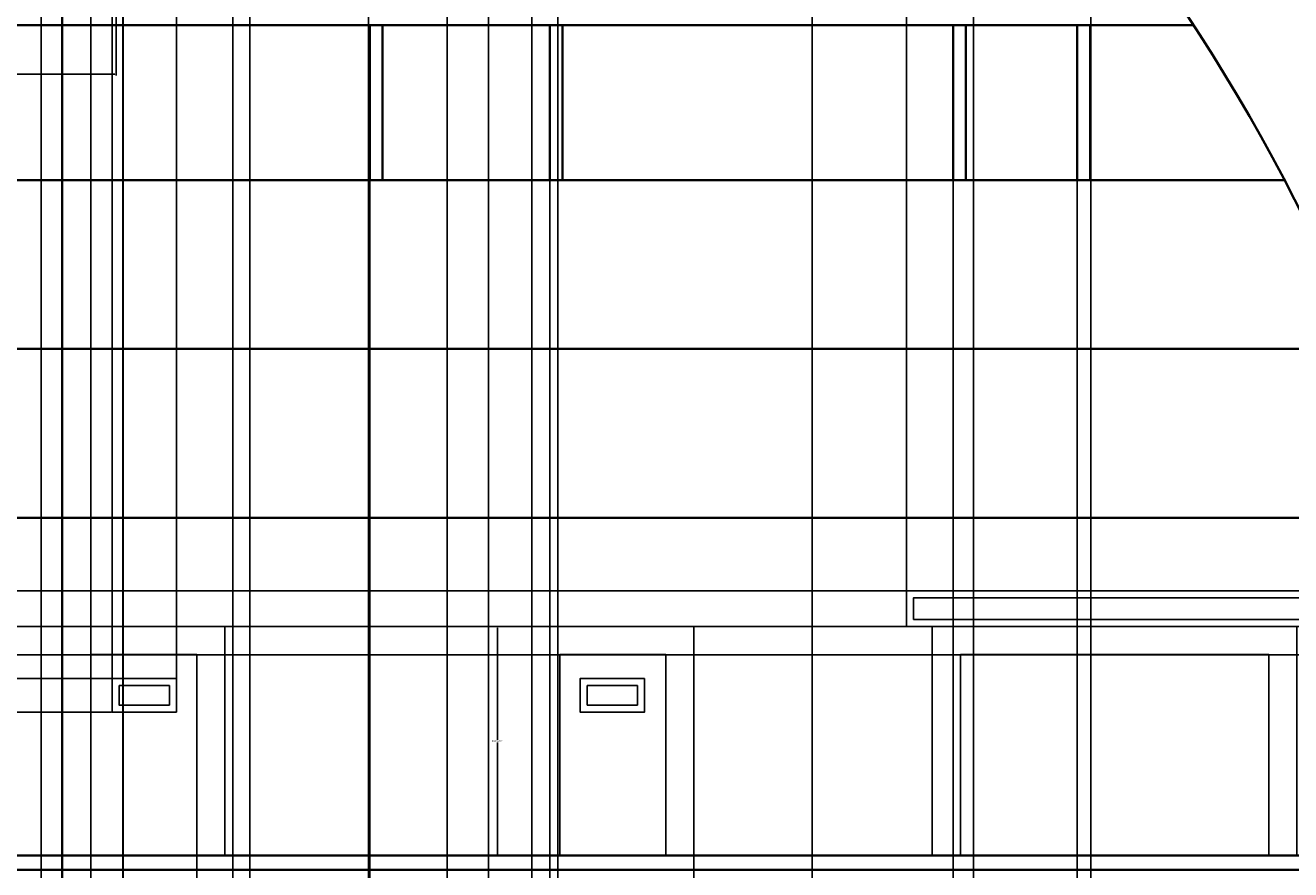
# Model space of a CAD drawing. Units: inches. Extents: x -19 to 408, y -26 to 603.
# Tile 3 of 7: x 137 to 317, y 169 to 289. Entities that reach past the tile are written whole.
import ezdxf

# ---------------------------------------------------------------- set-up
doc = ezdxf.new("R2010")
doc.units = ezdxf.units.IN
doc.header["$MEASUREMENT"] = 0
for name, color, linetype, lineweight in [('A-ANNO-DIMS', 2, 'Continuous', 18), ('A-DOOR', 3, 'Continuous', 25), ('A-ELEV', 7, 'Continuous', 35), ('A-GLAZ', 4, 'Continuous', 25)]:
    doc.layers.add(name, color=color, linetype=linetype, lineweight=lineweight)
doc.styles.get("Standard").update_dxf_attribs({"font": 'arial.ttf'})
doc.dimstyles.get("Standard").update_dxf_attribs({"dimtxt": 0.18, "dimasz": 0.18, "dimexe": 0.18, "dimexo": 0.0625, "dimgap": 0.09, "dimtad": 0, "dimtih": 1, "dimtoh": 1, "dimdec": 4, "dimzin": 0, "dimdsep": 46, "dimtxsty": 'Standard', "dimcen": 0.09, "dimadec": 0, "dimazin": 0, "dimtfac": 1, "dimtdec": 4, "dimtofl": 0, "dimtmove": 0, "dimatfit": 3, "dimfxl": 1, "dimtolj": 1, "dimtzin": 0, "dimarcsym": 0})

# ---------------------------------------------------------------- blocks, each defined once
blk = doc.blocks.new('WIN-1200')
for points in [[(0, 32.56), (59.66, 32.56), (59.66, 37.64), (0, 37.64)], [(1, 33.56), (58.66, 33.56), (58.66, 36.64), (1, 36.64)]]:
    blk.add_lwpolyline(points, close=True)
for points in [[(4.17, 0), (4.17, 32.56), (55.99, 32.56), (55.99, 0)], [(8.17, 0), (8.17, 28.56), (51.99, 28.56), (51.99, 0)]]:
    blk.add_lwpolyline(points)
blk = doc.blocks.new('DOOR-600')
for points in [[(0, 0), (0, 32.56), (23.06, 32.56), (23.06, 0)], [(4, 0), (4, 28.56), (19.06, 28.56), (19.06, 0)]]:
    blk.add_lwpolyline(points)
for points in [[(7.03, 25.16), (16.18, 25.16), (16.18, 20.4), (7.03, 20.4)], [(8.03, 24.16), (15.18, 24.16), (15.18, 21.4), (8.03, 21.4)]]:
    blk.add_lwpolyline(points, close=True)
blk = doc.blocks.new('RAIL-POST')
blk.add_lwpolyline([(0, 22), (1.83, 22), (1.83, 0), (0, 0)], close=True)
blk = doc.blocks.new('*D4')
at = {"layer": 'A-ANNO-DIMS', "color": 0, "lineweight": -2, "transparency": 16777216}
for p, q in [((89.99, 291.08), (89.99, 282.02)), ((149.65, 291.08), (149.65, 282.02)), ((90.17, 282.2), (118.7, 282.2)), ((149.47, 282.2), (120.94, 282.2))]:
    blk.add_line(p, q, dxfattribs=at)
at = {"layer": 'A-ANNO-DIMS', "color": 0, "transparency": 16777216}
for points in [[(90.17, 282.23), (90.17, 282.17), (89.99, 282.2)], [(149.47, 282.23), (149.47, 282.17), (149.65, 282.2)]]:
    blk.add_solid(points, dxfattribs=at)
at = {"layer": 'Defpoints', "color": 0, "transparency": 16777216}
for p in [(89.99, 291.15), (149.65, 291.15), (149.65, 282.2)]:
    blk.add_point(p, dxfattribs=at)
at = {"layer": 'A-ANNO-DIMS', "color": 0, "transparency": 16777216, "insert": (119.82, 282.2), "char_height": 0.18, "attachment_point": 5}
blk.add_mtext('\\A1;WINDOW 60 TYP.', dxfattribs=at)
blk = doc.blocks.new('*D6')
at = {"layer": 'A-ANNO-DIMS', "color": 0, "lineweight": -2, "transparency": 16777216}
for p, q in [((208.65, 203.7), (203.65, 203.7)), ((203.83, 203.52), (203.83, 187.61)), ((203.83, 171.33), (203.83, 187.24)), ((208.65, 171.15), (203.65, 171.15))]:
    blk.add_line(p, q, dxfattribs=at)
at = {"layer": 'A-ANNO-DIMS', "color": 0, "transparency": 16777216}
for points in [[(203.8, 203.52), (203.86, 203.52), (203.83, 203.7)], [(203.8, 171.33), (203.86, 171.33), (203.83, 171.15)]]:
    blk.add_solid(points, dxfattribs=at)
at = {"layer": 'Defpoints', "color": 0, "transparency": 16777216}
for p in [(203.83, 203.7), (208.71, 203.7), (208.71, 171.15)]:
    blk.add_point(p, dxfattribs=at)
at = {"layer": 'A-ANNO-DIMS', "color": 0, "transparency": 16777216, "insert": (203.83, 187.43), "char_height": 0.18, "attachment_point": 5}
blk.add_mtext('\\A1;DOOR 33 TYP.', dxfattribs=at)
blk = doc.blocks.new('*D7')
at = {"layer": 'A-ANNO-DIMS', "color": 0, "lineweight": -2, "transparency": 16777216}
for p, q in [((208.71, 171.08), (208.71, 166.08)), ((231.77, 171.08), (231.77, 166.08)), ((208.89, 166.26), (219.71, 166.26)), ((231.59, 166.26), (220.77, 166.26))]:
    blk.add_line(p, q, dxfattribs=at)
at = {"layer": 'A-ANNO-DIMS', "color": 0, "transparency": 16777216}
for points in [[(208.89, 166.29), (208.89, 166.23), (208.71, 166.26)], [(231.59, 166.29), (231.59, 166.23), (231.77, 166.26)]]:
    blk.add_solid(points, dxfattribs=at)
at = {"layer": 'Defpoints', "color": 0, "transparency": 16777216}
for p in [(208.71, 171.15), (231.77, 171.15), (208.71, 166.26)]:
    blk.add_point(p, dxfattribs=at)
at = {"layer": 'A-ANNO-DIMS', "color": 0, "transparency": 16777216, "insert": (220.24, 166.26), "char_height": 0.18, "attachment_point": 5}
blk.add_mtext('\\A1;23 TYP.', dxfattribs=at)
blk = doc.blocks.new('*D27')
at = {"layer": 'A-ANNO-DIMS', "color": 0, "lineweight": -2, "transparency": 16777216}
for p, q in [((288.17, 123.21), (288.17, 602.9)), ((288.35, 602.72), (324.05, 602.72)), ((360.39, 602.72), (324.69, 602.72)), ((360.57, 123.21), (360.57, 602.9))]:
    blk.add_line(p, q, dxfattribs=at)
at = {"layer": 'A-ANNO-DIMS', "color": 0, "transparency": 16777216}
for points in [[(288.35, 602.75), (288.35, 602.69), (288.17, 602.72)], [(360.39, 602.75), (360.39, 602.69), (360.57, 602.72)]]:
    blk.add_solid(points, dxfattribs=at)
at = {"layer": 'Defpoints', "color": 0, "transparency": 16777216}
for p in [(360.57, 602.72), (288.17, 123.15), (360.57, 123.15)]:
    blk.add_point(p, dxfattribs=at)
at = {"layer": 'A-ANNO-DIMS', "color": 0, "transparency": 16777216, "insert": (324.37, 602.72), "char_height": 0.18, "attachment_point": 5}
blk.add_mtext('\\A1;72.4', dxfattribs=at)
blk = doc.blocks.new('*D30')
at = {"layer": 'A-ANNO-DIMS', "color": 0, "lineweight": -2, "transparency": 16777216}
for p, q in [((360.57, 411.08), (360.57, -25.93)), ((185.52, 387.08), (185.52, -25.93)), ((185.7, -25.75), (272.59, -25.75)), ((360.39, -25.75), (273.5, -25.75))]:
    blk.add_line(p, q, dxfattribs=at)
at = {"layer": 'A-ANNO-DIMS', "color": 0, "transparency": 16777216}
for points in [[(185.7, -25.72), (185.7, -25.78), (185.52, -25.75)], [(360.39, -25.72), (360.39, -25.78), (360.57, -25.75)]]:
    blk.add_solid(points, dxfattribs=at)
at = {"layer": 'Defpoints', "color": 0, "transparency": 16777216}
for p in [(360.57, 411.15), (185.52, 387.15), (360.57, -25.75)]:
    blk.add_point(p, dxfattribs=at)
at = {"layer": 'A-ANNO-DIMS', "color": 0, "transparency": 16777216, "insert": (273.05, -25.75), "char_height": 0.18, "attachment_point": 5}
blk.add_mtext('\\A1;175.05', dxfattribs=at)
blk = doc.blocks.new('*D36')
at = {"layer": 'A-ANNO-DIMS', "color": 0, "lineweight": -2, "transparency": 16777216}
for p, q in [((52.15, 203.77), (52.15, 602.9)), ((52.33, 602.72), (96.69, 602.72)), ((141.84, 602.72), (97.48, 602.72)), ((142.02, 171.21), (142.02, 602.9))]:
    blk.add_line(p, q, dxfattribs=at)
at = {"layer": 'A-ANNO-DIMS', "color": 0, "transparency": 16777216}
for points in [[(52.33, 602.75), (52.33, 602.69), (52.15, 602.72)], [(141.84, 602.75), (141.84, 602.69), (142.02, 602.72)]]:
    blk.add_solid(points, dxfattribs=at)
at = {"layer": 'Defpoints', "color": 0, "transparency": 16777216}
for p in [(142.02, 602.72), (52.15, 203.7), (142.02, 171.15)]:
    blk.add_point(p, dxfattribs=at)
at = {"layer": 'A-ANNO-DIMS', "color": 0, "transparency": 16777216, "insert": (97.09, 602.72), "char_height": 0.18, "attachment_point": 5}
blk.add_mtext('\\A1;89.87', dxfattribs=at)
blk = doc.blocks.new('*D37')
at = {"layer": 'A-ANNO-DIMS', "color": 0, "lineweight": -2, "transparency": 16777216}
for p, q in [((142.02, 171.21), (142.02, 602.9)), ((142.2, 602.72), (174.97, 602.72)), ((208.53, 602.72), (175.76, 602.72)), ((208.71, 171.21), (208.71, 602.9))]:
    blk.add_line(p, q, dxfattribs=at)
at = {"layer": 'A-ANNO-DIMS', "color": 0, "transparency": 16777216}
for points in [[(142.2, 602.75), (142.2, 602.69), (142.02, 602.72)], [(208.53, 602.75), (208.53, 602.69), (208.71, 602.72)]]:
    blk.add_solid(points, dxfattribs=at)
at = {"layer": 'Defpoints', "color": 0, "transparency": 16777216}
for p in [(208.71, 602.72), (142.02, 171.15), (208.71, 171.15)]:
    blk.add_point(p, dxfattribs=at)
at = {"layer": 'A-ANNO-DIMS', "color": 0, "transparency": 16777216, "insert": (175.37, 602.72), "char_height": 0.18, "attachment_point": 5}
blk.add_mtext('\\A1;66.69', dxfattribs=at)
blk = doc.blocks.new('*D38')
at = {"layer": 'A-ANNO-DIMS', "color": 0, "lineweight": -2, "transparency": 16777216}
for p, q in [((208.71, 171.21), (208.71, 602.9)), ((208.89, 602.72), (234.95, 602.72)), ((261.81, 602.72), (235.74, 602.72)), ((261.99, 203.77), (261.99, 602.9))]:
    blk.add_line(p, q, dxfattribs=at)
at = {"layer": 'A-ANNO-DIMS', "color": 0, "transparency": 16777216}
for points in [[(208.89, 602.75), (208.89, 602.69), (208.71, 602.72)], [(261.81, 602.75), (261.81, 602.69), (261.99, 602.72)]]:
    blk.add_solid(points, dxfattribs=at)
at = {"layer": 'Defpoints', "color": 0, "transparency": 16777216}
for p in [(261.99, 602.72), (261.99, 203.7), (208.71, 171.15)]:
    blk.add_point(p, dxfattribs=at)
at = {"layer": 'A-ANNO-DIMS', "color": 0, "transparency": 16777216, "insert": (235.35, 602.72), "char_height": 0.18, "attachment_point": 5}
blk.add_mtext('\\A1;53.28', dxfattribs=at)
blk = doc.blocks.new('*D50')
at = {"layer": 'A-ANNO-DIMS', "color": 0, "lineweight": -2, "transparency": 16777216}
for p, q in [((104.21, 199.7), (407.65, 199.7)), ((407.47, 199.52), (407.47, 185.61)), ((407.47, 171.33), (407.47, 185.24)), ((104.21, 171.15), (407.65, 171.15))]:
    blk.add_line(p, q, dxfattribs=at)
at = {"layer": 'A-ANNO-DIMS', "color": 0, "transparency": 16777216}
for points in [[(407.44, 199.52), (407.5, 199.52), (407.47, 199.7)], [(407.44, 171.33), (407.5, 171.33), (407.47, 171.15)]]:
    blk.add_solid(points, dxfattribs=at)
at = {"layer": 'Defpoints', "color": 0, "transparency": 16777216}
for p in [(104.14, 199.7), (407.47, 199.7), (104.14, 171.15)]:
    blk.add_point(p, dxfattribs=at)
at = {"layer": 'A-ANNO-DIMS', "color": 0, "transparency": 16777216, "insert": (407.47, 185.43), "char_height": 0.18, "attachment_point": 5}
blk.add_mtext('\\A1;28.557', dxfattribs=at)
blk = doc.blocks.new('*D51')
at = {"layer": 'A-ANNO-DIMS', "color": 0, "lineweight": -2, "transparency": 16777216}
for p, q in [((108.207069, 203.703989), (407.651202, 203.703989)), ((407.471202, 203.523989), (407.471202, 201.883989)), ((407.471202, 199.883989), (407.471202, 201.523989)), ((104.207069, 199.703989), (407.651202, 199.703989))]:
    blk.add_line(p, q, dxfattribs=at)
at = {"layer": 'A-ANNO-DIMS', "color": 0, "transparency": 16777216}
for points in [[(407.441202, 203.523989), (407.501202, 203.523989), (407.471202, 203.703989)], [(407.441202, 199.883989), (407.501202, 199.883989), (407.471202, 199.703989)]]:
    blk.add_solid(points, dxfattribs=at)
at = {"layer": 'Defpoints', "color": 0, "transparency": 16777216}
for p in [(108.144569, 203.703989), (407.471202, 203.703989), (104.144569, 199.703989)]:
    blk.add_point(p, dxfattribs=at)
at = {"layer": 'A-ANNO-DIMS', "color": 0, "transparency": 16777216, "insert": (407.471202, 201.703989), "char_height": 0.18, "attachment_point": 5}
blk.add_mtext('\\A1;4', dxfattribs=at)
blk = doc.blocks.new('*D52')
at = {"layer": 'A-ANNO-DIMS', "color": 0, "lineweight": -2, "transparency": 16777216}
for p, q in [((111.87, 208.79), (407.65, 208.79)), ((407.47, 208.61), (407.47, 206.43)), ((407.47, 203.88), (407.47, 206.07)), ((111.87, 203.7), (407.65, 203.7))]:
    blk.add_line(p, q, dxfattribs=at)
at = {"layer": 'A-ANNO-DIMS', "color": 0, "transparency": 16777216}
for points in [[(407.44, 208.61), (407.5, 208.61), (407.47, 208.79)], [(407.44, 203.88), (407.5, 203.88), (407.47, 203.7)]]:
    blk.add_solid(points, dxfattribs=at)
at = {"layer": 'Defpoints', "color": 0, "transparency": 16777216}
for p in [(111.81, 208.79), (407.47, 208.79), (111.81, 203.7)]:
    blk.add_point(p, dxfattribs=at)
at = {"layer": 'A-ANNO-DIMS', "color": 0, "transparency": 16777216, "insert": (407.47, 206.25), "char_height": 0.18, "attachment_point": 5}
blk.add_mtext('\\A1;5.086', dxfattribs=at)
blk = doc.blocks.new('*D53')
at = {"layer": 'A-ANNO-DIMS', "color": 0, "lineweight": -2, "transparency": 16777216}
for p, q in [((142.02, 171.08), (142.02, -25.93)), ((146.02, 171.08), (146.02, -25.93)), ((142.2, -25.75), (143.87, -25.75)), ((145.84, -25.75), (144.18, -25.75))]:
    blk.add_line(p, q, dxfattribs=at)
at = {"layer": 'A-ANNO-DIMS', "color": 0, "transparency": 16777216}
for points in [[(142.2, -25.72), (142.2, -25.78), (142.02, -25.75)], [(145.84, -25.72), (145.84, -25.78), (146.02, -25.75)]]:
    blk.add_solid(points, dxfattribs=at)
at = {"layer": 'Defpoints', "color": 0, "transparency": 16777216}
for p in [(142.02, 171.15), (146.02, 171.15), (146.02, -25.75)]:
    blk.add_point(p, dxfattribs=at)
at = {"layer": 'A-ANNO-DIMS', "color": 0, "transparency": 16777216, "insert": (144.02, -25.75), "char_height": 0.18, "attachment_point": 5}
blk.add_mtext('\\A1;4', dxfattribs=at)
blk = doc.blocks.new('*D54')
at = {"layer": 'A-ANNO-DIMS', "color": 0, "lineweight": -2, "transparency": 16777216}
for p, q in [((146.02, 171.08), (146.02, -25.93)), ((161.09, 171.08), (161.09, -25.93)), ((146.2, -25.75), (153.1, -25.75)), ((160.91, -25.75), (154.01, -25.75))]:
    blk.add_line(p, q, dxfattribs=at)
at = {"layer": 'A-ANNO-DIMS', "color": 0, "transparency": 16777216}
for points in [[(146.2, -25.72), (146.2, -25.78), (146.02, -25.75)], [(160.91, -25.72), (160.91, -25.78), (161.09, -25.75)]]:
    blk.add_solid(points, dxfattribs=at)
at = {"layer": 'Defpoints', "color": 0, "transparency": 16777216}
for p in [(146.02, 171.15), (161.09, 171.15), (161.09, -25.75)]:
    blk.add_point(p, dxfattribs=at)
at = {"layer": 'A-ANNO-DIMS', "color": 0, "transparency": 16777216, "insert": (153.56, -25.75), "char_height": 0.18, "attachment_point": 5}
blk.add_mtext('\\A1;15.064', dxfattribs=at)
blk = doc.blocks.new('*D55')
at = {"layer": 'A-ANNO-DIMS', "color": 0, "lineweight": -2, "transparency": 16777216}
for p, q in [((146.02, 199.77), (146.02, 602.9)), ((146.2, 602.72), (147.14, 602.72)), ((148.87, 602.72), (147.93, 602.72)), ((149.05, 196.37), (149.05, 602.9))]:
    blk.add_line(p, q, dxfattribs=at)
at = {"layer": 'A-ANNO-DIMS', "color": 0, "transparency": 16777216}
for points in [[(146.2, 602.75), (146.2, 602.69), (146.02, 602.72)], [(148.87, 602.75), (148.87, 602.69), (149.05, 602.72)]]:
    blk.add_solid(points, dxfattribs=at)
at = {"layer": 'Defpoints', "color": 0, "transparency": 16777216}
for p in [(149.05, 602.72), (146.02, 199.7), (149.05, 196.31)]:
    blk.add_point(p, dxfattribs=at)
at = {"layer": 'A-ANNO-DIMS', "color": 0, "transparency": 16777216, "insert": (147.54, 602.72), "char_height": 0.18, "attachment_point": 5}
blk.add_mtext('\\A1;3.029', dxfattribs=at)
blk = doc.blocks.new('*D56')
at = {"layer": 'A-ANNO-DIMS', "color": 0, "lineweight": -2, "transparency": 16777216}
for p, q in [((149.05, 196.37), (149.05, 602.9)), ((149.23, 602.72), (153.3, 602.72)), ((158.02, 602.72), (153.95, 602.72)), ((158.2, 196.37), (158.2, 602.9))]:
    blk.add_line(p, q, dxfattribs=at)
at = {"layer": 'A-ANNO-DIMS', "color": 0, "transparency": 16777216}
for points in [[(149.23, 602.75), (149.23, 602.69), (149.05, 602.72)], [(158.02, 602.75), (158.02, 602.69), (158.2, 602.72)]]:
    blk.add_solid(points, dxfattribs=at)
at = {"layer": 'Defpoints', "color": 0, "transparency": 16777216}
for p in [(158.2, 602.72), (149.05, 196.31), (158.2, 196.31)]:
    blk.add_point(p, dxfattribs=at)
at = {"layer": 'A-ANNO-DIMS', "color": 0, "transparency": 16777216, "insert": (153.63, 602.72), "char_height": 0.18, "attachment_point": 5}
blk.add_mtext('\\A1;9.15', dxfattribs=at)
blk = doc.blocks.new('*D57')
at = {"layer": 'A-ANNO-DIMS', "color": 0, "lineweight": -2, "transparency": 16777216}
for p, q in [((148.99, 196.31), (-18.88, 196.31)), ((-18.7, 196.13), (-18.7, 194.11)), ((-18.7, 191.73), (-18.7, 193.75)), ((148.99, 191.55), (-18.88, 191.55))]:
    blk.add_line(p, q, dxfattribs=at)
at = {"layer": 'A-ANNO-DIMS', "color": 0, "transparency": 16777216}
for points in [[(-18.73, 196.13), (-18.67, 196.13), (-18.7, 196.31)], [(-18.73, 191.73), (-18.67, 191.73), (-18.7, 191.55)]]:
    blk.add_solid(points, dxfattribs=at)
at = {"layer": 'Defpoints', "color": 0, "transparency": 16777216}
for p in [(-18.7, 196.31), (149.05, 196.31), (149.05, 191.55)]:
    blk.add_point(p, dxfattribs=at)
at = {"layer": 'A-ANNO-DIMS', "color": 0, "transparency": 16777216, "insert": (-18.7, 193.93), "char_height": 0.18, "attachment_point": 5}
blk.add_mtext('\\A1;4.756', dxfattribs=at)
blk = doc.blocks.new('*D58')
at = {"layer": 'A-ANNO-DIMS', "color": 0, "lineweight": -2, "transparency": 16777216}
for p, q in [((145.96, 199.7), (-18.88, 199.7)), ((-18.7, 199.52), (-18.7, 198.19)), ((148.99, 196.31), (-18.88, 196.31)), ((-18.7, 196.49), (-18.7, 197.82))]:
    blk.add_line(p, q, dxfattribs=at)
at = {"layer": 'A-ANNO-DIMS', "color": 0, "transparency": 16777216}
for points in [[(-18.73, 199.52), (-18.67, 199.52), (-18.7, 199.7)], [(-18.73, 196.49), (-18.67, 196.49), (-18.7, 196.31)]]:
    blk.add_solid(points, dxfattribs=at)
at = {"layer": 'Defpoints', "color": 0, "transparency": 16777216}
for p in [(-18.7, 199.7), (146.02, 199.7), (149.05, 196.31)]:
    blk.add_point(p, dxfattribs=at)
at = {"layer": 'A-ANNO-DIMS', "color": 0, "transparency": 16777216, "insert": (-18.7, 198), "char_height": 0.18, "attachment_point": 5}
blk.add_mtext('\\A1;3.398', dxfattribs=at)
blk = doc.blocks.new('*D59')
at = {"layer": 'A-ANNO-DIMS', "color": 0, "lineweight": -2, "transparency": 16777216}
for p, q in [((161.15, 199.7), (407.65, 199.7)), ((407.47, 199.52), (407.47, 185.61)), ((407.47, 171.33), (407.47, 185.24)), ((161.15, 171.15), (407.65, 171.15))]:
    blk.add_line(p, q, dxfattribs=at)
at = {"layer": 'A-ANNO-DIMS', "color": 0, "transparency": 16777216}
for points in [[(407.44, 199.52), (407.5, 199.52), (407.47, 199.7)], [(407.44, 171.33), (407.5, 171.33), (407.47, 171.15)]]:
    blk.add_solid(points, dxfattribs=at)
at = {"layer": 'Defpoints', "color": 0, "transparency": 16777216}
for p in [(161.09, 199.7), (407.47, 199.7), (161.09, 171.15)]:
    blk.add_point(p, dxfattribs=at)
at = {"layer": 'A-ANNO-DIMS', "color": 0, "transparency": 16777216, "insert": (407.47, 185.43), "char_height": 0.18, "attachment_point": 5}
blk.add_mtext('\\A1;28.557', dxfattribs=at)
blk = doc.blocks.new('*D62')
at = {"layer": 'A-ANNO-DIMS', "color": 0, "lineweight": -2, "transparency": 16777216}
for p, q in [((131.96, 267.08), (131.96, -25.93)), ((185.68, 267.08), (185.68, -25.93)), ((132.14, -25.75), (158.43, -25.75)), ((185.5, -25.75), (159.21, -25.75))]:
    blk.add_line(p, q, dxfattribs=at)
at = {"layer": 'A-ANNO-DIMS', "color": 0, "transparency": 16777216}
for points in [[(132.14, -25.72), (132.14, -25.78), (131.96, -25.75)], [(185.5, -25.72), (185.5, -25.78), (185.68, -25.75)]]:
    blk.add_solid(points, dxfattribs=at)
at = {"layer": 'Defpoints', "color": 0, "transparency": 16777216}
for p in [(131.96, 267.15), (185.68, 267.15), (185.68, -25.75)]:
    blk.add_point(p, dxfattribs=at)
at = {"layer": 'A-ANNO-DIMS', "color": 0, "transparency": 16777216, "insert": (158.82, -25.75), "char_height": 0.18, "attachment_point": 5}
blk.add_mtext('\\A1;53.72', dxfattribs=at)
blk = doc.blocks.new('*D63')
at = {"layer": 'A-ANNO-DIMS', "color": 0, "lineweight": -2, "transparency": 16777216}
for p, q in [((185.68, 267.08), (185.68, -25.93)), ((211.27, 267.08), (211.27, -25.93)), ((185.86, -25.75), (198.01, -25.75)), ((211.09, -25.75), (198.94, -25.75))]:
    blk.add_line(p, q, dxfattribs=at)
at = {"layer": 'A-ANNO-DIMS', "color": 0, "transparency": 16777216}
for points in [[(185.86, -25.72), (185.86, -25.78), (185.68, -25.75)], [(211.09, -25.72), (211.09, -25.78), (211.27, -25.75)]]:
    blk.add_solid(points, dxfattribs=at)
at = {"layer": 'Defpoints', "color": 0, "transparency": 16777216}
for p in [(185.68, 267.15), (211.27, 267.15), (211.27, -25.75)]:
    blk.add_point(p, dxfattribs=at)
at = {"layer": 'A-ANNO-DIMS', "color": 0, "transparency": 16777216, "insert": (198.47, -25.75), "char_height": 0.18, "attachment_point": 5}
blk.add_mtext('\\A1;25.584', dxfattribs=at)
blk = doc.blocks.new('*D64')
at = {"layer": 'A-ANNO-DIMS', "color": 0, "lineweight": -2, "transparency": 16777216}
for p, q in [((211.27, 267.08), (211.27, -25.93)), ((268.61, 267.08), (268.61, -25.93)), ((211.45, -25.75), (239.55, -25.75)), ((268.43, -25.75), (240.33, -25.75))]:
    blk.add_line(p, q, dxfattribs=at)
at = {"layer": 'A-ANNO-DIMS', "color": 0, "transparency": 16777216}
for points in [[(211.45, -25.72), (211.45, -25.78), (211.27, -25.75)], [(268.43, -25.72), (268.43, -25.78), (268.61, -25.75)]]:
    blk.add_solid(points, dxfattribs=at)
at = {"layer": 'Defpoints', "color": 0, "transparency": 16777216}
for p in [(211.27, 267.15), (268.61, 267.15), (268.61, -25.75)]:
    blk.add_point(p, dxfattribs=at)
at = {"layer": 'A-ANNO-DIMS', "color": 0, "transparency": 16777216, "insert": (239.94, -25.75), "char_height": 0.18, "attachment_point": 5}
blk.add_mtext('\\A1;57.34', dxfattribs=at)
blk = doc.blocks.new('*D65')
at = {"layer": 'A-ANNO-DIMS', "color": 0, "lineweight": -2, "transparency": 16777216}
for p, q in [((268.61, 267.08), (268.61, -25.93)), ((286.26, 267.08), (286.26, -25.93)), ((268.79, -25.75), (276.98, -25.75)), ((286.08, -25.75), (277.89, -25.75))]:
    blk.add_line(p, q, dxfattribs=at)
at = {"layer": 'A-ANNO-DIMS', "color": 0, "transparency": 16777216}
for points in [[(268.79, -25.72), (268.79, -25.78), (268.61, -25.75)], [(286.08, -25.72), (286.08, -25.78), (286.26, -25.75)]]:
    blk.add_solid(points, dxfattribs=at)
at = {"layer": 'Defpoints', "color": 0, "transparency": 16777216}
for p in [(268.61, 267.15), (286.26, 267.15), (286.26, -25.75)]:
    blk.add_point(p, dxfattribs=at)
at = {"layer": 'A-ANNO-DIMS', "color": 0, "transparency": 16777216, "insert": (277.43, -25.75), "char_height": 0.18, "attachment_point": 5}
blk.add_mtext('\\A1;17.644', dxfattribs=at)
blk = doc.blocks.new('*D70')
at = {"layer": 'A-ANNO-DIMS', "color": 0, "lineweight": -2, "transparency": 16777216}
for p, q in [((150.62, 387.08), (150.62, -25.93)), ((185.52, 387.08), (185.52, -25.93)), ((150.8, -25.75), (167.6, -25.75)), ((185.34, -25.75), (168.53, -25.75))]:
    blk.add_line(p, q, dxfattribs=at)
at = {"layer": 'A-ANNO-DIMS', "color": 0, "transparency": 16777216}
for points in [[(150.8, -25.72), (150.8, -25.78), (150.62, -25.75)], [(185.34, -25.72), (185.34, -25.78), (185.52, -25.75)]]:
    blk.add_solid(points, dxfattribs=at)
at = {"layer": 'Defpoints', "color": 0, "transparency": 16777216}
for p in [(150.62, 387.15), (185.52, 387.15), (185.52, -25.75)]:
    blk.add_point(p, dxfattribs=at)
at = {"layer": 'A-ANNO-DIMS', "color": 0, "transparency": 16777216, "insert": (168.07, -25.75), "char_height": 0.18, "attachment_point": 5}
blk.add_mtext('\\A1;34.906', dxfattribs=at)
blk = doc.blocks.new('*D73')
at = {"layer": 'A-ANNO-DIMS', "color": 0, "lineweight": -2, "transparency": 16777216}
for p, q in [((185.52, 411.08), (185.52, -25.93)), ((208.71, 411.08), (208.71, -25.93)), ((185.7, -25.75), (196.72, -25.75)), ((208.53, -25.75), (197.51, -25.75))]:
    blk.add_line(p, q, dxfattribs=at)
at = {"layer": 'A-ANNO-DIMS', "color": 0, "transparency": 16777216}
for points in [[(185.7, -25.72), (185.7, -25.78), (185.52, -25.75)], [(208.53, -25.72), (208.53, -25.78), (208.71, -25.75)]]:
    blk.add_solid(points, dxfattribs=at)
at = {"layer": 'Defpoints', "color": 0, "transparency": 16777216}
for p in [(185.52, 411.15), (208.71, 411.15), (208.71, -25.75)]:
    blk.add_point(p, dxfattribs=at)
at = {"layer": 'A-ANNO-DIMS', "color": 0, "transparency": 16777216, "insert": (197.12, -25.75), "char_height": 0.18, "attachment_point": 5}
blk.add_mtext('\\A1;23.19', dxfattribs=at)
blk = doc.blocks.new('*D75')
at = {"layer": 'A-ANNO-DIMS', "color": 0, "lineweight": -2, "transparency": 16777216}
for p, q in [((212.43, 507.08), (212.43, -25.93)), ((248.57, 507.08), (248.57, -25.93)), ((212.61, -25.75), (230.11, -25.75)), ((248.39, -25.75), (230.89, -25.75))]:
    blk.add_line(p, q, dxfattribs=at)
at = {"layer": 'A-ANNO-DIMS', "color": 0, "transparency": 16777216}
for points in [[(212.61, -25.72), (212.61, -25.78), (212.43, -25.75)], [(248.39, -25.72), (248.39, -25.78), (248.57, -25.75)]]:
    blk.add_solid(points, dxfattribs=at)
at = {"layer": 'Defpoints', "color": 0, "transparency": 16777216}
for p in [(212.43, 507.15), (248.57, 507.15), (248.57, -25.75)]:
    blk.add_point(p, dxfattribs=at)
at = {"layer": 'A-ANNO-DIMS', "color": 0, "transparency": 16777216, "insert": (230.5, -25.75), "char_height": 0.18, "attachment_point": 5}
blk.add_mtext('\\A1;36.14', dxfattribs=at)
blk = doc.blocks.new('*D76')
at = {"layer": 'A-ANNO-DIMS', "color": 0, "lineweight": -2, "transparency": 16777216}
for p, q in [((248.57, 507.08), (248.57, -25.93)), ((271.51, 507.08), (271.51, -25.93)), ((248.75, -25.75), (259.58, -25.75)), ((271.33, -25.75), (260.51, -25.75))]:
    blk.add_line(p, q, dxfattribs=at)
at = {"layer": 'A-ANNO-DIMS', "color": 0, "transparency": 16777216}
for points in [[(248.75, -25.72), (248.75, -25.78), (248.57, -25.75)], [(271.33, -25.72), (271.33, -25.78), (271.51, -25.75)]]:
    blk.add_solid(points, dxfattribs=at)
at = {"layer": 'Defpoints', "color": 0, "transparency": 16777216}
for p in [(248.57, 507.15), (271.51, 507.15), (271.51, -25.75)]:
    blk.add_point(p, dxfattribs=at)
at = {"layer": 'A-ANNO-DIMS', "color": 0, "transparency": 16777216, "insert": (260.04, -25.75), "char_height": 0.18, "attachment_point": 5}
blk.add_mtext('\\A1;22.944', dxfattribs=at)
blk = doc.blocks.new('*D77')
at = {"layer": 'A-ANNO-DIMS', "color": 0, "lineweight": -2, "transparency": 16777216}
for p, q in [((271.51, 507.08), (271.51, -25.93)), ((325.24, 507.08), (325.24, -25.93)), ((271.69, -25.75), (297.98, -25.75)), ((325.06, -25.75), (298.77, -25.75))]:
    blk.add_line(p, q, dxfattribs=at)
at = {"layer": 'A-ANNO-DIMS', "color": 0, "transparency": 16777216}
for points in [[(271.69, -25.72), (271.69, -25.78), (271.51, -25.75)], [(325.06, -25.72), (325.06, -25.78), (325.24, -25.75)]]:
    blk.add_solid(points, dxfattribs=at)
at = {"layer": 'Defpoints', "color": 0, "transparency": 16777216}
for p in [(271.51, 507.15), (325.24, 507.15), (325.24, -25.75)]:
    blk.add_point(p, dxfattribs=at)
at = {"layer": 'A-ANNO-DIMS', "color": 0, "transparency": 16777216, "insert": (298.38, -25.75), "char_height": 0.18, "attachment_point": 5}
blk.add_mtext('\\A1;53.72', dxfattribs=at)
blk = doc.blocks.new('*D83')
at = {"layer": 'A-ANNO-DIMS', "color": 0, "lineweight": -2, "transparency": 16777216}
for p, q in [((141.92, 491.44), (141.92, -25.93)), ((166.23, 491.44), (166.23, -25.93)), ((142.1, -25.75), (153.69, -25.75)), ((166.05, -25.75), (154.45, -25.75))]:
    blk.add_line(p, q, dxfattribs=at)
at = {"layer": 'A-ANNO-DIMS', "color": 0, "transparency": 16777216}
for points in [[(142.1, -25.72), (142.1, -25.78), (141.92, -25.75)], [(166.05, -25.72), (166.05, -25.78), (166.23, -25.75)]]:
    blk.add_solid(points, dxfattribs=at)
at = {"layer": 'Defpoints', "color": 0, "transparency": 16777216}
for p in [(141.92, 491.5), (166.23, 491.5), (166.23, -25.75)]:
    blk.add_point(p, dxfattribs=at)
at = {"layer": 'A-ANNO-DIMS', "color": 0, "transparency": 16777216, "insert": (154.07, -25.75), "char_height": 0.18, "attachment_point": 5}
blk.add_mtext('\\A1;24.31', dxfattribs=at)
blk = doc.blocks.new('*D84')
at = {"layer": 'A-ANNO-DIMS', "color": 0, "lineweight": -2, "transparency": 16777216}
for p, q in [((138.97, 531.28), (138.97, -25.93)), ((168.64, 531.28), (168.64, -25.93)), ((139.15, -25.75), (153.41, -25.75)), ((168.46, -25.75), (154.2, -25.75))]:
    blk.add_line(p, q, dxfattribs=at)
at = {"layer": 'A-ANNO-DIMS', "color": 0, "transparency": 16777216}
for points in [[(139.15, -25.72), (139.15, -25.78), (138.97, -25.75)], [(168.46, -25.72), (168.46, -25.78), (168.64, -25.75)]]:
    blk.add_solid(points, dxfattribs=at)
at = {"layer": 'Defpoints', "color": 0, "transparency": 16777216}
for p in [(138.97, 531.34), (168.64, 531.34), (168.64, -25.75)]:
    blk.add_point(p, dxfattribs=at)
at = {"layer": 'A-ANNO-DIMS', "color": 0, "transparency": 16777216, "insert": (153.81, -25.75), "char_height": 0.18, "attachment_point": 5}
blk.add_mtext('\\A1;29.67', dxfattribs=at)
blk = doc.blocks.new('*D95')
at = {"layer": 'A-ANNO-DIMS', "color": 0, "lineweight": -2, "transparency": 16777216}
for p, q in [((150.57, 85.97), (150.57, 602.9)), ((150.75, 602.72), (173.31, 602.72)), ((196.49, 602.72), (173.93, 602.72)), ((196.67, 85.97), (196.67, 602.9))]:
    blk.add_line(p, q, dxfattribs=at)
at = {"layer": 'A-ANNO-DIMS', "color": 0, "transparency": 16777216}
for points in [[(150.75, 602.75), (150.75, 602.69), (150.57, 602.72)], [(196.49, 602.75), (196.49, 602.69), (196.67, 602.72)]]:
    blk.add_solid(points, dxfattribs=at)
at = {"layer": 'Defpoints', "color": 0, "transparency": 16777216}
for p in [(196.67, 602.72), (150.57, 85.9), (196.67, 85.9)]:
    blk.add_point(p, dxfattribs=at)
at = {"layer": 'A-ANNO-DIMS', "color": 0, "transparency": 16777216, "insert": (173.62, 602.72), "char_height": 0.18, "attachment_point": 5}
blk.add_mtext('\\A1;46.1', dxfattribs=at)
blk = doc.blocks.new('*D96')
at = {"layer": 'A-ANNO-DIMS', "color": 0, "lineweight": -2, "transparency": 16777216}
for p, q in [((196.67, 85.97), (196.67, 602.9)), ((196.85, 602.72), (199.31, 602.72)), ((202.41, 602.72), (199.96, 602.72)), ((202.59, 85.97), (202.59, 602.9))]:
    blk.add_line(p, q, dxfattribs=at)
at = {"layer": 'A-ANNO-DIMS', "color": 0, "transparency": 16777216}
for points in [[(196.85, 602.75), (196.85, 602.69), (196.67, 602.72)], [(202.41, 602.75), (202.41, 602.69), (202.59, 602.72)]]:
    blk.add_solid(points, dxfattribs=at)
at = {"layer": 'Defpoints', "color": 0, "transparency": 16777216}
for p in [(202.59, 602.72), (196.67, 85.9), (202.59, 85.9)]:
    blk.add_point(p, dxfattribs=at)
at = {"layer": 'A-ANNO-DIMS', "color": 0, "transparency": 16777216, "insert": (199.63, 602.72), "char_height": 0.18, "attachment_point": 5}
blk.add_mtext('\\A1;5.92', dxfattribs=at)
blk = doc.blocks.new('*D106')
at = {"layer": 'A-ANNO-DIMS', "color": 0, "lineweight": -2, "transparency": 16777216}
for p, q in [((106.54, 387.08), (106.54, -25.93)), ((185.52, 387.08), (185.52, -25.93)), ((106.72, -25.75), (145.64, -25.75)), ((185.34, -25.75), (146.43, -25.75))]:
    blk.add_line(p, q, dxfattribs=at)
at = {"layer": 'A-ANNO-DIMS', "color": 0, "transparency": 16777216}
for points in [[(106.72, -25.72), (106.72, -25.78), (106.54, -25.75)], [(185.34, -25.72), (185.34, -25.78), (185.52, -25.75)]]:
    blk.add_solid(points, dxfattribs=at)
at = {"layer": 'Defpoints', "color": 0, "transparency": 16777216}
for p in [(106.54, 387.15), (185.52, 387.15), (106.54, -25.75)]:
    blk.add_point(p, dxfattribs=at)
at = {"layer": 'A-ANNO-DIMS', "color": 0, "transparency": 16777216, "insert": (146.03, -25.75), "char_height": 0.18, "attachment_point": 5}
blk.add_mtext('\\A1;78.98', dxfattribs=at)

msp = doc.modelspace()

# ---------------------------------------------------------------- linework, layer by layer
at = {"layer": 'A-ELEV'}
for p, q in [((84.1933, 289.1472), (302.7917, 289.1472)), ((87.7217, 267.1472), (315.7238, 267.1472)), ((326.6715, 243.1472), (98.524, 243.1472)), ((98.524, 243.1472), (326.6715, 243.1472)), ((36.5712, 219.1472), (334.2819, 219.1472)), ((36.5712, 171.1472), (337.2261, 171.1472)), ((165.088, 171.1472), (142.0243, 171.1472)), ((36.5712, 169.1472), (336.868, 169.1472))]:
    msp.add_line(p, q, dxfattribs=at)
msp.add_ellipse((188.4962, 355.8525), major_axis=(71.2607, 129.8447), ratio=0.58959924, start_param=6.80188927, end_param=9.63162337, dxfattribs=at)
at = {"layer": 'A-ELEV', "extrusion": (0, 0, -1)}
msp.add_ellipse((217.8094, 257.6617), major_axis=(99.7631, -123.1178), ratio=0.55109141, start_param=3.84421936, end_param=6.63412911, dxfattribs=at)

# ---------------------------------------------------------------- block references
at = {"layer": 'A-DOOR'}
msp.add_blockref('DOOR-600', (142.024, 171.147), dxfattribs=at)
at = {"layer": 'A-DOOR', "extrusion": (0, 0, -1), "zscale": -1}
msp.add_blockref('DOOR-600', (-231.7733, 171.147), dxfattribs=at)
at = {"layer": 'A-ELEV'}
for p in [(185.6825, 267.147), (211.2668, 267.147), (268.611, 267.147), (286.2553, 267.147)]:
    msp.add_blockref('RAIL-POST', p, dxfattribs=at)
at = {"layer": 'A-GLAZ', "extrusion": (0, 0, -1), "zscale": -1}
msp.add_blockref('WIN-1200', (-321.6443, 171.147), dxfattribs=at)

# ---------------------------------------------------------------- dimensions: what is measured, and where the dimension line sits
at = {"layer": 'A-ANNO-DIMS'}
for base, p1, p2, override, picture, middle in [((142.0243, 602.7184), (52.1528, 203.704), (142.0243, 171.1472), {"dimdec": 2, "dimlfac": 1, "dimrnd": 0, "dimzin": 0, "dimdsep": 46, "dimlunit": 2}, '*D36', (97.0885, 602.7184)), ((208.70929, 602.71845), (142.02426, 171.14723), (208.70929, 171.14723), {"dimdec": 2, "dimlfac": 1, "dimrnd": 0, "dimzin": 0, "dimdsep": 46, "dimlunit": 2}, '*D37', (175.36677, 602.71845)), ((149.0532, 602.7184), (146.0243, 199.704), (149.0532, 196.3059), {"dimdec": 3, "dimlfac": 1, "dimrnd": 0, "dimzin": 0, "dimdsep": 46, "dimlunit": 2}, '*D55', (147.5387, 602.7184)), ((158.2025, 602.7184), (149.0532, 196.3059), (158.2025, 196.3059), {"dimdec": 2, "dimlfac": 1, "dimrnd": 0, "dimzin": 0, "dimdsep": 46, "dimlunit": 2}, '*D56', (153.6278, 602.7184)), ((196.6731, 602.7184), (150.5712, 85.9033), (196.6731, 85.9033), {"dimdec": 1, "dimlfac": 1, "dimrnd": 0, "dimzin": 0, "dimdsep": 46, "dimlunit": 2}, '*D95', (173.6222, 602.7184)), ((202.5934, 602.7184), (196.6731, 85.9033), (202.5934, 85.9033), {"dimdec": 2, "dimlfac": 1, "dimrnd": 0, "dimzin": 0, "dimdsep": 46, "dimlunit": 2}, '*D96', (199.6333, 602.7184)), ((261.9882, 602.7184), (208.7093, 171.1472), (261.9882, 203.704), {"dimdec": 2, "dimlfac": 1, "dimrnd": 0, "dimzin": 0, "dimdsep": 46, "dimlunit": 2}, '*D38', (235.3487, 602.7184)), ((360.5712, 602.7184), (288.1664, 123.1472), (360.5712, 123.1472), {"dimdec": 1, "dimlfac": 1, "dimrnd": 0, "dimzin": 0, "dimdsep": 46, "dimlunit": 2}, '*D27', (324.3688, 602.7184)), ((168.6421, -25.7528), (138.9724, 531.3421), (168.6421, 531.3421), {"dimdec": 2, "dimlfac": 1, "dimrnd": 0, "dimzin": 0, "dimdsep": 46, "dimlunit": 2}, '*D84', (153.8072, -25.7528)), ((248.5703, -25.7528), (212.4303, 507.1472), (248.5703, 507.1472), {"dimdec": 2, "dimlfac": 1, "dimrnd": 0, "dimzin": 0, "dimdsep": 46, "dimlunit": 2}, '*D75', (230.5003, -25.7528)), ((271.514, -25.7528), (248.5703, 507.1472), (271.514, 507.1472), {"dimdec": 3, "dimlfac": 1, "dimrnd": 0, "dimzin": 0, "dimdsep": 46, "dimlunit": 2}, '*D76', (260.0422, -25.7528)), ((325.2366, -25.7528), (271.514, 507.1472), (325.2366, 507.1472), {"dimdec": 2, "dimlfac": 1, "dimrnd": 0, "dimzin": 0, "dimdsep": 46, "dimlunit": 2}, '*D77', (298.3753, -25.7528)), ((166.228, -25.7528), (141.9163, 491.5037), (166.228, 491.5037), {"dimdec": 2, "dimlfac": 1, "dimrnd": 0, "dimzin": 0, "dimdsep": 46, "dimlunit": 2}, '*D83', (154.0722, -25.7528)), ((360.5712, -25.7528), (185.5212, 387.1472), (360.5712, 411.1472), {"dimdec": 2, "dimlfac": 1, "dimrnd": 0, "dimzin": 0, "dimdsep": 46, "dimlunit": 2}, '*D30', (273.0462, -25.7528)), ((208.7093, -25.7528), (185.5212, 411.1472), (208.7093, 411.1472), {"dimdec": 2, "dimlfac": 1, "dimrnd": 0, "dimzin": 0, "dimdsep": 46, "dimlunit": 2}, '*D73', (197.1153, -25.7528)), ((106.5444, -25.7528), (185.5212, 387.1472), (106.5444, 387.1472), {"dimdec": 2, "dimlfac": 1, "dimrnd": 0, "dimzin": 0, "dimdsep": 46, "dimlunit": 2}, '*D106', (146.0328, -25.7528)), ((185.5212, -25.7528), (150.6152, 387.1472), (185.5212, 387.1472), {"dimdec": 3, "dimlfac": 1, "dimrnd": 0, "dimzin": 0, "dimdsep": 46, "dimlunit": 2}, '*D70', (168.0682, -25.7528)), ((185.6827, -25.7528), (131.9601, 267.1472), (185.6827, 267.1472), {"dimdec": 2, "dimlfac": 1, "dimrnd": 0, "dimzin": 0, "dimdsep": 46, "dimlunit": 2}, '*D62', (158.8214, -25.7528)), ((211.267, -25.7528), (185.6827, 267.1472), (211.267, 267.1472), {"dimdec": 3, "dimlfac": 1, "dimrnd": 0, "dimzin": 0, "dimdsep": 46, "dimlunit": 2}, '*D63', (198.4749, -25.7528)), ((268.6112, -25.7528), (211.267, 267.1472), (268.6112, 267.1472), {"dimdec": 2, "dimlfac": 1, "dimrnd": 0, "dimzin": 0, "dimdsep": 46, "dimlunit": 2}, '*D64', (239.9391, -25.7528)), ((286.2555, -25.7528), (268.6112, 267.1472), (286.2555, 267.1472), {"dimdec": 3, "dimlfac": 1, "dimrnd": 0, "dimzin": 0, "dimdsep": 46, "dimlunit": 2}, '*D65', (277.4333, -25.7528)), ((146.0243, -25.7528), (142.0243, 171.1472), (146.0243, 171.1472), {"dimdec": 0, "dimlfac": 1, "dimrnd": 0, "dimzin": 0, "dimdsep": 46, "dimlunit": 2}, '*D53', (144.0243, -25.7528)), ((161.088, -25.7528), (146.0243, 171.1472), (161.088, 171.1472), {"dimdec": 3, "dimlfac": 1, "dimrnd": 0, "dimzin": 0, "dimdsep": 46, "dimlunit": 2}, '*D54', (153.5561, -25.7528))]:
    dim = msp.add_linear_dim(base=base, p1=p1, p2=p2, dimstyle='Standard', override=override, dxfattribs=at)
    dim.commit()
    dim.dimension.update_dxf_attribs({"geometry": picture, "text_midpoint": middle})
dim = msp.add_linear_dim(base=(149.6464, 282.1988), p1=(89.9901, 291.1472), p2=(149.6464, 291.1472), text='WINDOW <> TYP.', dimstyle='Standard', override={"dimdec": 0, "dimlfac": 1, "dimrnd": 0, "dimzin": 0, "dimdsep": 46, "dimlunit": 2}, dxfattribs=at)
dim.commit()
dim.dimension.update_dxf_attribs({"geometry": '*D4', "text_midpoint": (119.8182, 282.1988)})
for base, p1, p2, override, picture, middle in [((407.4712, 208.7903), (111.8091, 203.704), (111.8091, 208.7903), {"dimdec": 3, "dimlfac": 1, "dimrnd": 0, "dimzin": 0, "dimdsep": 46, "dimlunit": 2}, '*D52', (407.4712, 206.2471)), ((407.4712, 203.704), (104.1446, 199.704), (108.1446, 203.704), {"dimdec": 0, "dimlfac": 1, "dimrnd": 0, "dimzin": 0, "dimdsep": 46, "dimlunit": 2}, '*D51', (407.4712, 201.704)), ((-18.698, 199.704), (149.0532, 196.3059), (146.0243, 199.704), {"dimdec": 3, "dimlfac": 1, "dimrnd": 0, "dimzin": 0, "dimdsep": 46, "dimlunit": 2}, '*D58', (-18.698, 198.0049)), ((407.4712, 199.704), (104.1446, 171.1472), (104.1446, 199.704), {"dimdec": 3, "dimlfac": 1, "dimrnd": 0, "dimzin": 0, "dimdsep": 46, "dimlunit": 2}, '*D50', (407.4712, 185.4256)), ((407.4712, 199.704), (161.088, 171.1472), (161.088, 199.704), {"dimdec": 3, "dimlfac": 1, "dimrnd": 0, "dimzin": 0, "dimdsep": 46, "dimlunit": 2}, '*D59', (407.4712, 185.4256)), ((-18.698, 196.3059), (149.0532, 191.5497), (149.0532, 196.3059), {"dimdec": 3, "dimlfac": 1, "dimrnd": 0, "dimzin": 0, "dimdsep": 46, "dimlunit": 2}, '*D57', (-18.698, 193.9278))]:
    dim = msp.add_linear_dim(base=base, p1=p1, p2=p2, angle=90, dimstyle='Standard', override=override, dxfattribs=at)
    dim.commit()
    dim.dimension.update_dxf_attribs({"geometry": picture, "text_midpoint": middle})
for base, p1, p2, angle, text, picture, middle in [((203.8258, 203.704), (208.7093, 171.1472), (208.7093, 203.704), 90, 'DOOR <> TYP.', '*D6', (203.8258, 187.4256)), ((208.7093, 166.2637), (231.773, 171.1472), (208.7093, 171.1472), 180, '<> TYP.', '*D7', (220.2411, 166.2637))]:
    dim = msp.add_linear_dim(base=base, p1=p1, p2=p2, angle=angle, text=text, dimstyle='Standard', override={"dimdec": 0, "dimlfac": 1, "dimrnd": 0, "dimzin": 0, "dimdsep": 46, "dimlunit": 2}, dxfattribs=at)
    dim.commit()
    dim.dimension.update_dxf_attribs({"geometry": picture, "text_midpoint": middle})

doc.saveas('drawing.dxf')
